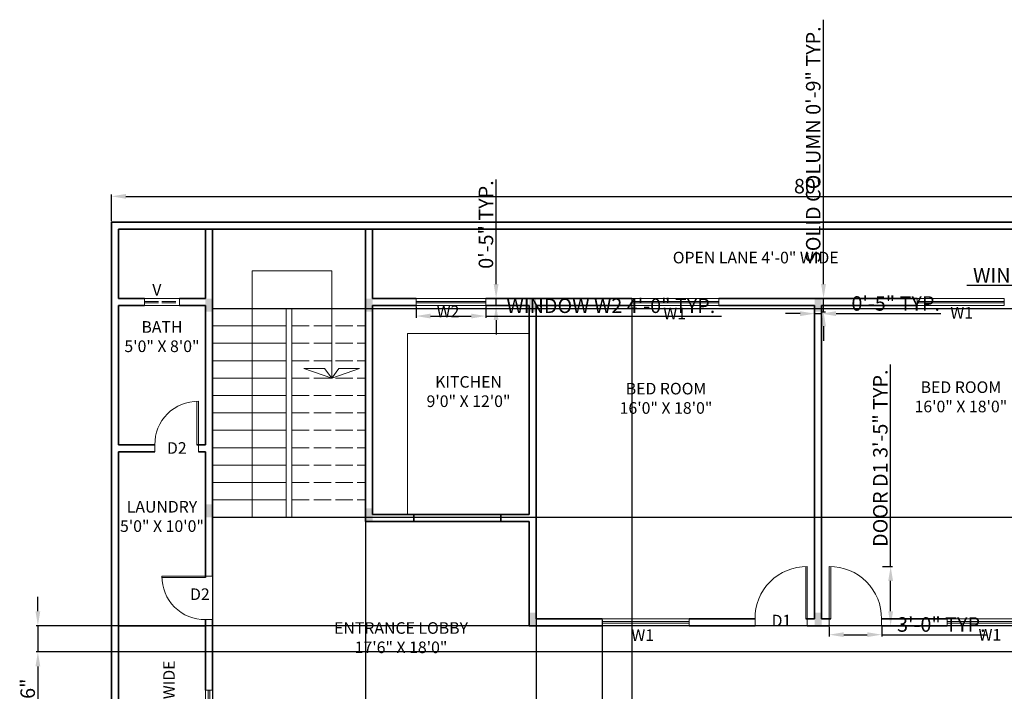
# Model space of a CAD drawing. Units: inches. Extents: x 13878 to 15021, y 3891 to 4810.
# Tile 2 of 3: x 13897 to 14576, y 4347 to 4810. Entities that reach past the tile are written whole.
import ezdxf

# ---------------------------------------------------------------- set-up
doc = ezdxf.new("R2010")
doc.units = ezdxf.units.IN
doc.linetypes.add('ACAD_ISO02W100', pattern=[15, 12, -3])
for name, color, linetype, lineweight in [('A-ANNO-DIMS', 2, 'Continuous', 18), ('A-ANNO-TEXT', 7, 'Continuous', 18), ('A-AREA-IDEN', 7, 'Continuous', 18), ('A-COLS-PATT', 7, 'Continuous', 18), ('A-DOOR', 4, 'Continuous', 18), ('A-FLOR-FIXT', 8, 'Continuous', 18), ('A-FLOR-STRS', 220, 'Continuous', 18), ('A-FLOR-STRS-OVHD', 220, 'ACAD_ISO02W100', 18), ('A-GLAZ', 4, 'Continuous', 18), ('A-GLAZ-HIDN', 4, 'ACAD_ISO02W100', 13), ('A-WALL', 150, 'Continuous', 35), ('C-SITE-WALL', 150, 'Continuous', 35)]:
    doc.layers.add(name, color=color, linetype=linetype, lineweight=lineweight)
doc.styles.get("Standard").update_dxf_attribs({"font": 'arial.ttf'})
doc.dimstyles.new('ISO-25', dxfattribs={"dimtxt": 10, "dimasz": 10, "dimexe": 1.25, "dimexo": 0.625, "dimtad": 1, "dimdec": 0, "dimlunit": 3, "dimtxsty": 'Standard', "dimcen": 2.5, "dimadec": 0, "dimazin": 0, "dimtfac": 1, "dimtdec": 0, "dimtmove": 0, "dimatfit": 3, "dimfxl": 1, "dimarcsym": 0})

# ---------------------------------------------------------------- blocks, each defined once
blk = doc.blocks.new('*D7')
at = {"layer": 'A-ANNO-DIMS', "color": 0, "lineweight": -2, "transparency": 16777216}
for p, q in [((13960.64, 4671.28), (13960.64, 4689.65)), ((13970.64, 4688.4), (14910.64, 4688.4)), ((14920.64, 4671.28), (14920.64, 4689.65))]:
    blk.add_line(p, q, dxfattribs=at)
at = {"layer": 'A-ANNO-DIMS', "color": 0, "transparency": 16777216}
for points in [[(13970.64, 4690.07), (13970.64, 4686.74), (13960.64, 4688.4)], [(14910.64, 4690.07), (14910.64, 4686.74), (14920.64, 4688.4)]]:
    blk.add_solid(points, dxfattribs=at)
at = {"layer": 'Defpoints', "color": 0, "transparency": 16777216}
for p in [(14920.64, 4688.4), (13960.64, 4670.66), (14920.64, 4670.66)]:
    blk.add_point(p, dxfattribs=at)
at = {"layer": 'A-ANNO-DIMS', "color": 0, "transparency": 16777216, "insert": (14440.64, 4694.14), "char_height": 10, "attachment_point": 5}
blk.add_mtext("80'", dxfattribs=at)
blk = doc.blocks.new('DOOR-D1-36IN')
for p, q in [((0, 4.8), (0, 40.8)), ((1, 4.8), (1, 40.8)), ((0, 4.8), (0, 0)), ((36, 4.8), (36, 0))]:
    blk.add_line(p, q)
blk.add_arc((0.5, 5.3), 35.5, 359.19307, 90.80693)
blk = doc.blocks.new('DOOR-D2-30IN')
for p, q in [((0, 30), (4.8, 30)), ((0, 0), (4.8, 0)), ((4.8, 1), (34.8, 1)), ((4.8, 0), (34.8, 0))]:
    blk.add_line(p, q)
blk.add_arc((5.3, 0.5), 29.5, 359.02898, 90.97102)
blk = doc.blocks.new('WINDOW-W1-60IN')
for p, q in [((0, 0), (0, 4.8)), ((0, 4.8), (60, 4.8)), ((0, 2.9), (60, 2.9)), ((0, 1.9), (60, 1.9)), ((60, 0), (60, 4.8)), ((0, 0), (60, 0))]:
    blk.add_line(p, q)
blk = doc.blocks.new('WINDOW-W2-48IN')
for p, q in [((0, 0), (0, 4.8)), ((0, 4.8), (48, 4.8)), ((0, 2.9), (48, 2.9)), ((0, 1.9), (48, 1.9)), ((48, 0), (48, 4.8)), ((0, 0), (48, 0))]:
    blk.add_line(p, q)
blk = doc.blocks.new('COLUMN-RECT-SOLID')
h = blk.add_hatch(color=256)
h.dxf.hatch_style = 1
h.paths.add_polyline_path([(0, 0), (4.8, 0), (4.8, 9), (0, 9)])
blk = doc.blocks.new('VENT-FRAME-24IN')
for p, q in [((0, 0), (0, 4.8)), ((0, 4.8), (24, 4.8)), ((24, 0), (24, 4.8)), ((0, 0), (24, 0))]:
    blk.add_line(p, q)
blk = doc.blocks.new('*D18')
at = {"layer": 'A-ANNO-DIMS', "color": 0, "lineweight": -2, "ltscale": 2, "transparency": 16777216}
for p, q in [((14451.59, 4627.86), (14451.59, 4810.24)), ((14450.86, 4617.86), (14452.84, 4617.86)), ((14451.59, 4608.86), (14451.59, 4617.86)), ((14450.86, 4608.86), (14452.84, 4608.86)), ((14451.59, 4598.86), (14451.59, 4588.86))]:
    blk.add_line(p, q, dxfattribs=at)
at = {"layer": 'A-ANNO-DIMS', "color": 0, "ltscale": 2, "transparency": 16777216}
for points in [[(14449.92, 4627.86), (14453.25, 4627.86), (14451.59, 4617.86)], [(14449.92, 4598.86), (14453.25, 4598.86), (14451.59, 4608.86)]]:
    blk.add_solid(points, dxfattribs=at)
at = {"layer": 'Defpoints', "color": 0, "ltscale": 2, "transparency": 16777216}
for p in [(14450.24, 4617.86), (14451.59, 4617.86), (14450.24, 4608.86)]:
    blk.add_point(p, dxfattribs=at)
at = {"layer": 'A-ANNO-DIMS', "color": 0, "ltscale": 2, "transparency": 16777216, "insert": (14445.79, 4724.05), "char_height": 10, "attachment_point": 5, "rotation": 90}
blk.add_mtext('SOLID COLUMN 0\'-9" TYP.', dxfattribs=at)
blk = doc.blocks.new('*D19')
at = {"layer": 'A-ANNO-DIMS', "color": 0, "lineweight": -2, "ltscale": 2, "transparency": 16777216}
for p, q in [((14435.44, 4607.51), (14425.44, 4607.51)), ((14445.44, 4608.23), (14445.44, 4606.26)), ((14445.44, 4607.51), (14450.24, 4607.51)), ((14450.24, 4608.23), (14450.24, 4606.26)), ((14460.24, 4607.51), (14532.44, 4607.51))]:
    blk.add_line(p, q, dxfattribs=at)
at = {"layer": 'A-ANNO-DIMS', "color": 0, "ltscale": 2, "transparency": 16777216}
for points in [[(14435.44, 4609.18), (14435.44, 4605.84), (14445.44, 4607.51)], [(14460.24, 4609.18), (14460.24, 4605.84), (14450.24, 4607.51)]]:
    blk.add_solid(points, dxfattribs=at)
at = {"layer": 'Defpoints', "color": 0, "ltscale": 2, "transparency": 16777216}
for p in [(14445.44, 4608.86), (14450.24, 4608.86), (14450.24, 4607.51)]:
    blk.add_point(p, dxfattribs=at)
at = {"layer": 'A-ANNO-DIMS', "color": 0, "ltscale": 2, "transparency": 16777216, "insert": (14501.34, 4613.24), "char_height": 10, "attachment_point": 5}
blk.add_mtext('0\'-5" TYP.', dxfattribs=at)
blk = doc.blocks.new('*D24')
at = {"layer": 'A-ANNO-DIMS', "color": 0, "lineweight": -2, "ltscale": 2, "transparency": 16777216}
for p, q in [((14713.04, 4626.86), (14550.41, 4626.86)), ((14713.04, 4618.48), (14713.04, 4628.11)), ((14763.04, 4626.86), (14723.04, 4626.86)), ((14773.04, 4618.48), (14773.04, 4628.11))]:
    blk.add_line(p, q, dxfattribs=at)
at = {"layer": 'A-ANNO-DIMS', "color": 0, "ltscale": 2, "transparency": 16777216}
for points in [[(14723.04, 4628.53), (14723.04, 4625.19), (14713.04, 4626.86)], [(14763.04, 4628.53), (14763.04, 4625.19), (14773.04, 4626.86)]]:
    blk.add_solid(points, dxfattribs=at)
at = {"layer": 'Defpoints', "color": 0, "ltscale": 2, "transparency": 16777216}
for p in [(14713.04, 4626.86), (14713.04, 4617.86), (14773.04, 4617.86)]:
    blk.add_point(p, dxfattribs=at)
at = {"layer": 'A-ANNO-DIMS', "color": 0, "ltscale": 2, "transparency": 16777216, "insert": (14626.72, 4632.66), "char_height": 10, "attachment_point": 5}
blk.add_mtext('WINDOW W1 5\'-0" TYP.', dxfattribs=at)
blk = doc.blocks.new('*D26')
at = {"layer": 'A-ANNO-DIMS', "color": 0, "lineweight": -2, "ltscale": 2, "transparency": 16777216}
for p, q in [((14170.64, 4612.43), (14170.64, 4604.61)), ((14218.64, 4612.43), (14218.64, 4604.61)), ((14180.64, 4605.86), (14208.64, 4605.86)), ((14218.64, 4605.86), (14381.27, 4605.86))]:
    blk.add_line(p, q, dxfattribs=at)
at = {"layer": 'A-ANNO-DIMS', "color": 0, "ltscale": 2, "transparency": 16777216}
for points in [[(14180.64, 4607.53), (14180.64, 4604.19), (14170.64, 4605.86)], [(14208.64, 4607.53), (14208.64, 4604.19), (14218.64, 4605.86)]]:
    blk.add_solid(points, dxfattribs=at)
at = {"layer": 'Defpoints', "color": 0, "ltscale": 2, "transparency": 16777216}
for p in [(14170.64, 4613.06), (14218.64, 4613.06), (14218.64, 4605.86)]:
    blk.add_point(p, dxfattribs=at)
at = {"layer": 'A-ANNO-DIMS', "color": 0, "ltscale": 2, "transparency": 16777216, "insert": (14304.95, 4611.66), "char_height": 10, "attachment_point": 5}
blk.add_mtext('WINDOW W2 4\'-0" TYP.', dxfattribs=at)
blk = doc.blocks.new('*D27')
at = {"layer": 'A-ANNO-DIMS', "color": 0, "lineweight": -2, "ltscale": 2, "transparency": 16777216}
for p, q in [((14225.84, 4627.86), (14225.84, 4700.06)), ((14219.26, 4617.86), (14227.09, 4617.86)), ((14225.84, 4613.06), (14225.84, 4617.86)), ((14219.26, 4613.06), (14227.09, 4613.06)), ((14225.84, 4603.06), (14225.84, 4593.06))]:
    blk.add_line(p, q, dxfattribs=at)
at = {"layer": 'A-ANNO-DIMS', "color": 0, "ltscale": 2, "transparency": 16777216}
for points in [[(14224.17, 4627.86), (14227.5, 4627.86), (14225.84, 4617.86)], [(14224.17, 4603.06), (14227.5, 4603.06), (14225.84, 4613.06)]]:
    blk.add_solid(points, dxfattribs=at)
at = {"layer": 'Defpoints', "color": 0, "ltscale": 2, "transparency": 16777216}
for p in [(14218.64, 4617.86), (14225.84, 4617.86), (14218.64, 4613.06)]:
    blk.add_point(p, dxfattribs=at)
at = {"layer": 'A-ANNO-DIMS', "color": 0, "ltscale": 2, "transparency": 16777216, "insert": (14220.11, 4668.96), "char_height": 10, "attachment_point": 5, "rotation": 90}
blk.add_mtext('0\'-5" TYP.', dxfattribs=at)
blk = doc.blocks.new('*D30')
at = {"layer": 'A-ANNO-DIMS', "color": 0, "lineweight": -2, "ltscale": 2, "transparency": 16777216}
for p, q in [((14497.86, 4433.19), (14497.86, 4572.43)), ((14492.34, 4433.19), (14499.11, 4433.19)), ((14497.86, 4402.26), (14497.86, 4423.19)), ((14492.34, 4392.26), (14499.11, 4392.26))]:
    blk.add_line(p, q, dxfattribs=at)
at = {"layer": 'A-ANNO-DIMS', "color": 0, "ltscale": 2, "transparency": 16777216}
for points in [[(14496.19, 4423.19), (14499.52, 4423.19), (14497.86, 4433.19)], [(14496.19, 4402.26), (14499.52, 4402.26), (14497.86, 4392.26)]]:
    blk.add_solid(points, dxfattribs=at)
at = {"layer": 'Defpoints', "color": 0, "ltscale": 2, "transparency": 16777216}
for p in [(14491.72, 4433.19), (14497.86, 4433.19), (14491.72, 4392.26)]:
    blk.add_point(p, dxfattribs=at)
at = {"layer": 'A-ANNO-DIMS', "color": 0, "ltscale": 2, "transparency": 16777216, "insert": (14492.05, 4507.81), "char_height": 10, "attachment_point": 5, "rotation": 90}
blk.add_mtext('DOOR D1 3\'-5" TYP.', dxfattribs=at)
blk = doc.blocks.new('*D31')
at = {"layer": 'A-ANNO-DIMS', "color": 0, "lineweight": -2, "ltscale": 2, "transparency": 16777216}
for p, q in [((14455.58, 4391.63), (14455.58, 4384.87)), ((14465.58, 4386.12), (14481.72, 4386.12)), ((14491.72, 4391.63), (14491.72, 4384.87)), ((14491.72, 4386.12), (14563.91, 4386.12))]:
    blk.add_line(p, q, dxfattribs=at)
at = {"layer": 'A-ANNO-DIMS', "color": 0, "ltscale": 2, "transparency": 16777216}
for points in [[(14465.58, 4387.79), (14465.58, 4384.45), (14455.58, 4386.12)], [(14481.72, 4387.79), (14481.72, 4384.45), (14491.72, 4386.12)]]:
    blk.add_solid(points, dxfattribs=at)
at = {"layer": 'Defpoints', "color": 0, "ltscale": 2, "transparency": 16777216}
for p in [(14455.58, 4392.26), (14491.72, 4392.26), (14491.72, 4386.12)]:
    blk.add_point(p, dxfattribs=at)
at = {"layer": 'A-ANNO-DIMS', "color": 0, "ltscale": 2, "transparency": 16777216, "insert": (14532.81, 4391.85), "char_height": 10, "attachment_point": 5}
blk.add_mtext('3\'-0" TYP.', dxfattribs=at)
blk = doc.blocks.new('*D36')
at = {"layer": 'A-ANNO-DIMS', "color": 0, "lineweight": -2, "ltscale": 2, "transparency": 16777216}
for p, q in [((14030.24, 4466.43), (14030.24, 3898.66)), ((14135.84, 4466.43), (14135.84, 3898.66)), ((14040.24, 3899.91), (14125.84, 3899.91))]:
    blk.add_line(p, q, dxfattribs=at)
at = {"layer": 'A-ANNO-DIMS', "color": 0, "ltscale": 2, "transparency": 16777216}
for points in [[(14040.24, 3901.58), (14040.24, 3898.24), (14030.24, 3899.91)], [(14125.84, 3901.58), (14125.84, 3898.24), (14135.84, 3899.91)]]:
    blk.add_solid(points, dxfattribs=at)
at = {"layer": 'Defpoints', "color": 0, "ltscale": 2, "transparency": 16777216}
for p in [(14030.24, 4467.06), (14135.84, 4467.06), (14135.84, 3899.91)]:
    blk.add_point(p, dxfattribs=at)
at = {"layer": 'A-ANNO-DIMS', "color": 0, "ltscale": 2, "transparency": 16777216, "insert": (14083.04, 3905.71), "char_height": 10, "attachment_point": 5}
blk.add_mtext('8\'-9 1/2"', dxfattribs=at)
blk = doc.blocks.new('*D37')
at = {"layer": 'A-ANNO-DIMS', "color": 0, "lineweight": -2, "ltscale": 2, "transparency": 16777216}
for p, q in [((14030.86, 4611.06), (14972.64, 4611.06)), ((14971.39, 4477.06), (14971.39, 4601.06)), ((14030.86, 4467.06), (14972.64, 4467.06))]:
    blk.add_line(p, q, dxfattribs=at)
at = {"layer": 'A-ANNO-DIMS', "color": 0, "ltscale": 2, "transparency": 16777216}
for points in [[(14969.72, 4601.06), (14973.05, 4601.06), (14971.39, 4611.06)], [(14969.72, 4477.06), (14973.05, 4477.06), (14971.39, 4467.06)]]:
    blk.add_solid(points, dxfattribs=at)
at = {"layer": 'Defpoints', "color": 0, "ltscale": 2, "transparency": 16777216}
for p in [(14030.24, 4611.06), (14971.39, 4611.06), (14030.24, 4467.06)]:
    blk.add_point(p, dxfattribs=at)
at = {"layer": 'A-ANNO-DIMS', "color": 0, "ltscale": 2, "transparency": 16777216, "insert": (14965.66, 4539.06), "char_height": 10, "attachment_point": 5, "rotation": 90}
blk.add_mtext('12\'-0"', dxfattribs=at)
blk = doc.blocks.new('*D38')
at = {"layer": 'A-ANNO-DIMS', "color": 0, "lineweight": -2, "ltscale": 2, "transparency": 16777216}
for p, q in [((14253.44, 4612.43), (14253.44, 3898.66)), ((14319.44, 4612.43), (14319.44, 3898.66)), ((14263.44, 3899.91), (14309.44, 3899.91))]:
    blk.add_line(p, q, dxfattribs=at)
at = {"layer": 'A-ANNO-DIMS', "color": 0, "ltscale": 2, "transparency": 16777216}
for points in [[(14263.44, 3901.58), (14263.44, 3898.24), (14253.44, 3899.91)], [(14309.44, 3901.58), (14309.44, 3898.24), (14319.44, 3899.91)]]:
    blk.add_solid(points, dxfattribs=at)
at = {"layer": 'Defpoints', "color": 0, "ltscale": 2, "transparency": 16777216}
for p in [(14253.44, 4613.06), (14319.44, 4613.06), (14319.44, 3899.91)]:
    blk.add_point(p, dxfattribs=at)
at = {"layer": 'A-ANNO-DIMS', "color": 0, "ltscale": 2, "transparency": 16777216, "insert": (14286.44, 3905.64), "char_height": 10, "attachment_point": 5}
blk.add_mtext('5\'-6"', dxfattribs=at)
blk = doc.blocks.new('*D39')
at = {"layer": 'A-ANNO-DIMS', "color": 0, "lineweight": -2, "ltscale": 2, "transparency": 16777216}
for p, q in [((14253.44, 4396.43), (14253.44, 3898.66)), ((14298.9, 4396.43), (14298.9, 3898.66)), ((14263.44, 3899.91), (14288.9, 3899.91)), ((14298.9, 3899.91), (14360.03, 3899.91))]:
    blk.add_line(p, q, dxfattribs=at)
at = {"layer": 'A-ANNO-DIMS', "color": 0, "ltscale": 2, "transparency": 16777216}
for points in [[(14263.44, 3901.58), (14263.44, 3898.24), (14253.44, 3899.91)], [(14288.9, 3901.58), (14288.9, 3898.24), (14298.9, 3899.91)]]:
    blk.add_solid(points, dxfattribs=at)
at = {"layer": 'Defpoints', "color": 0, "ltscale": 2, "transparency": 16777216}
for p in [(14253.44, 4397.06), (14298.9, 4397.06), (14298.9, 3899.91)]:
    blk.add_point(p, dxfattribs=at)
at = {"layer": 'A-ANNO-DIMS', "color": 0, "ltscale": 2, "transparency": 16777216, "insert": (14334.46, 3905.71), "char_height": 10, "attachment_point": 5}
blk.add_mtext('3\'-9 1/2"', dxfattribs=at)
blk = doc.blocks.new('*D40')
at = {"layer": 'A-ANNO-DIMS', "color": 0, "lineweight": -2, "ltscale": 2, "transparency": 16777216}
for p, q in [((13909.89, 4402.26), (13909.89, 4412.26)), ((14838.41, 4392.26), (13908.64, 4392.26)), ((13909.89, 4392.26), (13909.89, 4374.26)), ((14838.41, 4374.26), (13908.64, 4374.26)), ((13909.89, 4364.26), (13909.89, 4327.37))]:
    blk.add_line(p, q, dxfattribs=at)
at = {"layer": 'A-ANNO-DIMS', "color": 0, "ltscale": 2, "transparency": 16777216}
for points in [[(13908.22, 4402.26), (13911.55, 4402.26), (13909.89, 4392.26)], [(13908.22, 4364.26), (13911.55, 4364.26), (13909.89, 4374.26)]]:
    blk.add_solid(points, dxfattribs=at)
at = {"layer": 'Defpoints', "color": 0, "ltscale": 2, "transparency": 16777216}
for p in [(14839.04, 4392.26), (13909.89, 4374.26), (14839.04, 4374.26)]:
    blk.add_point(p, dxfattribs=at)
at = {"layer": 'A-ANNO-DIMS', "color": 0, "ltscale": 2, "transparency": 16777216, "insert": (13904.16, 4340.81), "char_height": 10, "attachment_point": 5, "rotation": 90}
blk.add_mtext('1\'-6"', dxfattribs=at)

msp = doc.modelspace()

# ---------------------------------------------------------------- linework, layer by layer
at = {"layer": 'A-FLOR-FIXT'}
for q in [(14164.64, 4469.06), (14248.64, 4593.86)]:
    msp.add_line((14164.64, 4593.86), q, dxfattribs=at)
at = {"layer": 'A-FLOR-STRS'}
for p, q in [((14057.64, 4467.06), (14057.64, 4637.01)), ((14057.64, 4637.01), (14112.49, 4637.01)), ((14112.49, 4637.01), (14112.49, 4563.06)), ((14030.24, 4611.06), (14085.04, 4611.06)), ((14081.04, 4611.06), (14081.04, 4467.06)), ((14085.04, 4611.06), (14085.04, 4467.06)), ((14030.24, 4599.06), (14081.04, 4599.06)), ((14030.24, 4587.06), (14081.04, 4587.06)), ((14030.24, 4575.06), (14081.04, 4575.06)), ((14112.49, 4563.06), (14093.25, 4569.62)), ((14093.25, 4569.62), (14107.6, 4569.62)), ((14112.49, 4563.06), (14107.6, 4569.62)), ((14112.49, 4563.06), (14131.72, 4569.62)), ((14112.49, 4563.06), (14117.37, 4569.62)), ((14131.72, 4569.62), (14117.37, 4569.62)), ((14030.24, 4563.06), (14081.04, 4563.06)), ((14030.24, 4551.06), (14081.04, 4551.06)), ((14030.24, 4539.06), (14081.04, 4539.06)), ((14030.24, 4527.06), (14081.04, 4527.06)), ((14030.24, 4515.06), (14081.04, 4515.06)), ((14030.24, 4503.06), (14081.04, 4503.06)), ((14030.24, 4491.06), (14081.04, 4491.06)), ((14030.24, 4479.06), (14081.04, 4479.06)), ((14030.24, 4467.06), (14085.04, 4467.06))]:
    msp.add_line(p, q, dxfattribs=at)
at = {"layer": 'A-FLOR-STRS-OVHD'}
for p, q in [((14085.04, 4611.06), (14135.84, 4611.06)), ((14085.04, 4599.06), (14135.84, 4599.06)), ((14085.04, 4587.06), (14135.84, 4587.06)), ((14085.04, 4575.06), (14135.84, 4575.06)), ((14085.04, 4563.06), (14135.84, 4563.06)), ((14085.04, 4551.06), (14135.84, 4551.06)), ((14085.04, 4539.06), (14135.84, 4539.06)), ((14085.04, 4527.06), (14135.84, 4527.06)), ((14085.04, 4515.06), (14135.84, 4515.06)), ((14085.04, 4503.06), (14135.84, 4503.06)), ((14085.04, 4491.06), (14135.84, 4491.06)), ((14085.04, 4479.06), (14135.84, 4479.06)), ((14085.04, 4467.06), (14135.84, 4467.06))]:
    msp.add_line(p, q, dxfattribs=at)
at = {"layer": 'A-GLAZ-HIDN', "ltscale": 0.8}
for p, q in [((13983.44, 4615.96), (14007.44, 4615.96)), ((13983.44, 4614.96), (14007.44, 4614.96))]:
    msp.add_line(p, q, dxfattribs=at)
at = {"layer": 'A-WALL'}
for p, q in [((14025.44, 4617.86), (14025.44, 4665.86)), ((14030.24, 4617.86), (14030.24, 4665.86)), ((14135.84, 4617.86), (14135.84, 4665.86)), ((14140.64, 4617.86), (14140.64, 4665.86)), ((13965.44, 4617.86), (13983.44, 4617.86)), ((14007.44, 4617.86), (14025.44, 4617.86)), ((14030.24, 4426.5), (14030.24, 4617.86)), ((14135.84, 4617.86), (14135.84, 4464.26)), ((14140.64, 4617.86), (14170.64, 4617.86)), ((14218.64, 4617.86), (14319.44, 4617.86)), ((14379.44, 4617.86), (14516.24, 4617.86)), ((13965.44, 4613.06), (13983.44, 4613.06)), ((14007.44, 4613.06), (14025.44, 4613.06)), ((14025.44, 4517.06), (14025.44, 4613.06)), ((14140.64, 4613.06), (14140.64, 4469.06)), ((14140.64, 4613.06), (14170.64, 4613.06)), ((14218.64, 4613.06), (14248.64, 4613.06)), ((14248.64, 4613.06), (14248.64, 4469.06)), ((14253.44, 4613.06), (14253.44, 4397.06)), ((14253.44, 4613.06), (14319.44, 4613.06)), ((14379.44, 4613.06), (14445.44, 4613.06)), ((14445.44, 4613.06), (14445.44, 4397.06)), ((14450.24, 4613.06), (14450.24, 4397.06)), ((14450.24, 4613.06), (14516.24, 4613.06)), ((13965.44, 4517.06), (13990.54, 4517.06)), ((14019.54, 4517.06), (14025.44, 4517.06)), ((13965.44, 4512.26), (13990.54, 4512.26)), ((14020.54, 4512.26), (14025.44, 4512.26)), ((14025.44, 4425.5), (14025.44, 4512.26)), ((14140.64, 4469.06), (14169.09, 4469.06)), ((14169.09, 4469.06), (14169.09, 4464.26)), ((14169.09, 4469.06), (14229.09, 4469.06)), ((14229.09, 4469.06), (14229.09, 4464.26)), ((14229.09, 4469.06), (14248.64, 4469.06)), ((14135.84, 4464.26), (14169.09, 4464.26)), ((14169.09, 4464.26), (14229.09, 4464.26)), ((14229.09, 4464.26), (14248.64, 4464.26)), ((14248.64, 4464.26), (14248.64, 4392.26)), ((14025.44, 4392.26), (14025.44, 4396.5)), ((14030.24, 4347.86), (14030.24, 4396.5)), ((14253.44, 4397.06), (14298.9, 4397.06)), ((14358.9, 4397.06), (14404.36, 4397.06)), ((14439.36, 4397.06), (14445.44, 4397.06)), ((14450.24, 4397.06), (14456.58, 4397.06)), ((14491.58, 4397.06), (14536.91, 4397.06)), ((13965.44, 4392.26), (14025.44, 4392.26)), ((14025.44, 4347.86), (14025.44, 4392.26)), ((14248.64, 4392.26), (14298.9, 4392.26)), ((14358.9, 4392.26), (14404.36, 4392.26)), ((14440.36, 4392.26), (14445.44, 4392.26)), ((14445.44, 4392.26), (14455.58, 4392.26)), ((14491.58, 4392.26), (14536.91, 4392.26))]:
    msp.add_line(p, q, dxfattribs=at)
at = {"layer": 'C-SITE-WALL'}
for p, q in [((13960.64, 4670.66), (14920.64, 4670.66)), ((13960.64, 3950.66), (13960.64, 4670.66)), ((13965.44, 4665.86), (14839.04, 4665.86)), ((13965.44, 4617.86), (13965.44, 4665.86)), ((13965.44, 4517.06), (13965.44, 4613.06)), ((13965.44, 4392.26), (13965.44, 4512.26)), ((13965.44, 3956.66), (13965.44, 4392.26))]:
    msp.add_line(p, q, dxfattribs=at)

# ---------------------------------------------------------------- block references
at = {"layer": 'A-COLS-PATT'}
for p in [(14025.44, 4608.86), (14135.84, 4608.86), (14248.64, 4608.86), (14445.44, 4608.86), (14025.44, 4467.07), (14135.84, 4464.27), (14248.64, 4392.26), (14445.44, 4392.26)]:
    msp.add_blockref('COLUMN-RECT-SOLID', p, dxfattribs=at)
at = {"layer": 'A-DOOR'}
for p, rotation in [((14020.55, 4512.26), 90.00000000000733), ((14030.24, 4426.5), 180)]:
    msp.add_blockref('DOOR-D2-30IN', p, dxfattribs=dict(at, rotation=rotation))
at = {"layer": 'A-DOOR', "extrusion": (0, 0, -1), "zscale": -1}
msp.add_blockref('DOOR-D1-36IN', (-14440.36, 4392.26), dxfattribs=at)
at = {"layer": 'A-DOOR'}
msp.add_blockref('DOOR-D1-36IN', (14455.58, 4392.26), dxfattribs=at)
at = {"layer": 'A-GLAZ'}
for name, p in [('VENT-FRAME-24IN', (13983.44, 4613.06)), ('WINDOW-W2-48IN', (14170.64, 4613.06)), ('WINDOW-W1-60IN', (14319.44, 4613.06))]:
    msp.add_blockref(name, p, dxfattribs=at)
for p, rotation in [((14576.24, 4617.86), 180), ((14358.9, 4397.06), 180), ((14596.91, 4397.06), 180), ((14030.24, 4287.86), 89.99999999999301)]:
    msp.add_blockref('WINDOW-W1-60IN', p, dxfattribs=dict(at, rotation=rotation))

# ---------------------------------------------------------------- texts
at = {"layer": 'A-ANNO-TEXT', "char_height": 8, "attachment_point": 1}
for s, insert in [('V', (13988.76, 4627.96)), ('W2', (14184.87, 4613.06)), ('W1', (14341.12, 4611.69)), ('W1', (14539.02, 4612.08)), ('D2', (13998.88, 4518.86)), ('D2', (14014.79, 4418.03)), ('D1', (14415.78, 4399.82)), ('W1', (14319.1, 4389.75)), ('W1', (14558.47, 4390))]:
    msp.add_mtext_dynamic_manual_height_columns(s, width=16.3853, gutter_width=12.5, heights=[0], dxfattribs=dict(at, insert=insert))
at = {"layer": 'A-AREA-IDEN', "char_height": 8, "attachment_point": 1}
for s, width, insert in [('OPEN LANE 4\'-0" WIDE', 379.1288, (14347.64, 4650.18)), ('\\pxqc;BATH\\P5\'0" X 8\'0"', 60, (13965.44, 4602.35)), ('\\pxqc;KITCHEN\\P9\'0" X 12\'0"', 60, (14176.81, 4564.46)), ('\\pxqc;BED ROOM\\P16\'0" X 18\'0"', 65.572, (14310.2, 4559.8)), ('\\pxqc;BED ROOM\\P16\'0" X 18\'0"', 65.572, (14513.52, 4560.81)), ('\\pxqc;LAUNDRY\\P5\'0" X 10\'0"', 60, (13965.44, 4478.33)), ('\\pxqc;ENTRANCE LOBBY\\P17\'6" X 18\'0"', 129.4248, (14095.57, 4394.72))]:
    msp.add_mtext_dynamic_manual_height_columns(s, width=width, gutter_width=12.5, heights=[0], dxfattribs=dict(at, insert=insert))
at = {"layer": 'A-AREA-IDEN', "insert": (13996.3, 4253.96), "char_height": 8, "attachment_point": 1, "rotation": 90}
msp.add_mtext_dynamic_manual_height_columns('OPEN LANE 5\'-0" WIDE', width=379.1288, gutter_width=12.5, heights=[0], dxfattribs=at)

# ---------------------------------------------------------------- dimensions: what is measured, and where the dimension line sits
at = {"layer": 'A-ANNO-DIMS', "ltscale": 2}
for base, p1, p2, angle, text, picture, middle in [((14451.59, 4617.86), (14450.24, 4608.86), (14450.24, 4617.86), 90, 'SOLID COLUMN <> TYP.', '*D18', (14445.79, 4724.05)), ((14225.84, 4617.86), (14218.64, 4613.06), (14218.64, 4617.86), 90, '<> TYP.', '*D27', (14220.11, 4668.96)), ((14713.04, 4626.86), (14773.04, 4617.86), (14713.04, 4617.86), 180, 'WINDOW W1 <> TYP.', '*D24', (14626.72, 4632.66)), ((14497.86, 4433.19), (14491.72, 4392.26), (14491.72, 4433.19), 90, 'DOOR D1 <> TYP.', '*D30', (14492.05, 4507.81))]:
    dim = msp.add_linear_dim(base=base, p1=p1, p2=p2, angle=angle, text=text, dimstyle='ISO-25', override={"dimdec": 1, "dimlfac": 1, "dimrnd": 0, "dimzin": 1, "dimdsep": 46, "dimlunit": 4, "dimfrac": 2}, dxfattribs=at)
    dim.commit()
    dim.dimension.update_dxf_attribs({"geometry": picture, "text_midpoint": middle})
at = {"layer": 'A-ANNO-DIMS'}
dim = msp.add_linear_dim(base=(14920.64, 4688.4), p1=(13960.64, 4670.66), p2=(14920.64, 4670.66), dimstyle='ISO-25', override={"dimclrd": 0, "dimclre": 0, "dimclrt": 0}, dxfattribs=at)
dim.commit()
dim.dimension.update_dxf_attribs({"geometry": '*D7', "text_midpoint": (14440.64, 4694.14)})
at = {"layer": 'A-ANNO-DIMS', "ltscale": 2}
for base, p1, p2, text, picture, middle in [((14218.64, 4605.86), (14170.64, 4613.06), (14218.64, 4613.06), 'WINDOW W2 <> TYP.', '*D26', (14304.95, 4611.66)), ((14450.24, 4607.51), (14445.44, 4608.86), (14450.24, 4608.86), '<> TYP.', '*D19', (14501.34, 4613.24)), ((14491.72, 4386.12), (14455.58, 4392.26), (14491.72, 4392.26), '<> TYP.', '*D31', (14532.81, 4391.85))]:
    dim = msp.add_linear_dim(base=base, p1=p1, p2=p2, text=text, dimstyle='ISO-25', override={"dimdec": 1, "dimlfac": 1, "dimrnd": 0, "dimzin": 1, "dimdsep": 46, "dimlunit": 4, "dimfrac": 2}, dxfattribs=at)
    dim.commit()
    dim.dimension.update_dxf_attribs({"geometry": picture, "text_midpoint": middle})
for base, p1, p2, picture, middle in [((14971.39, 4611.06), (14030.24, 4467.06), (14030.24, 4611.06), '*D37', (14965.66, 4539.06)), ((13909.89, 4374.26), (14839.04, 4392.26), (14839.04, 4374.26), '*D40', (13904.16, 4340.81))]:
    dim = msp.add_linear_dim(base=base, p1=p1, p2=p2, angle=90, dimstyle='ISO-25', override={"dimdec": 1, "dimlfac": 1, "dimrnd": 0, "dimzin": 1, "dimdsep": 46, "dimlunit": 4, "dimfrac": 2}, dxfattribs=at)
    dim.commit()
    dim.dimension.update_dxf_attribs({"geometry": picture, "text_midpoint": middle})
for base, p1, p2, picture, middle in [((14319.44, 3899.91), (14253.44, 4613.06), (14319.44, 4613.06), '*D38', (14286.44, 3905.64)), ((14135.84, 3899.91), (14030.24, 4467.06), (14135.84, 4467.06), '*D36', (14083.04, 3905.71)), ((14298.9, 3899.91), (14253.44, 4397.06), (14298.9, 4397.06), '*D39', (14334.46, 3905.71))]:
    dim = msp.add_linear_dim(base=base, p1=p1, p2=p2, dimstyle='ISO-25', override={"dimdec": 1, "dimlfac": 1, "dimrnd": 0, "dimzin": 1, "dimdsep": 46, "dimlunit": 4, "dimfrac": 2}, dxfattribs=at)
    dim.commit()
    dim.dimension.update_dxf_attribs({"geometry": picture, "text_midpoint": middle})

doc.saveas('drawing.dxf')
